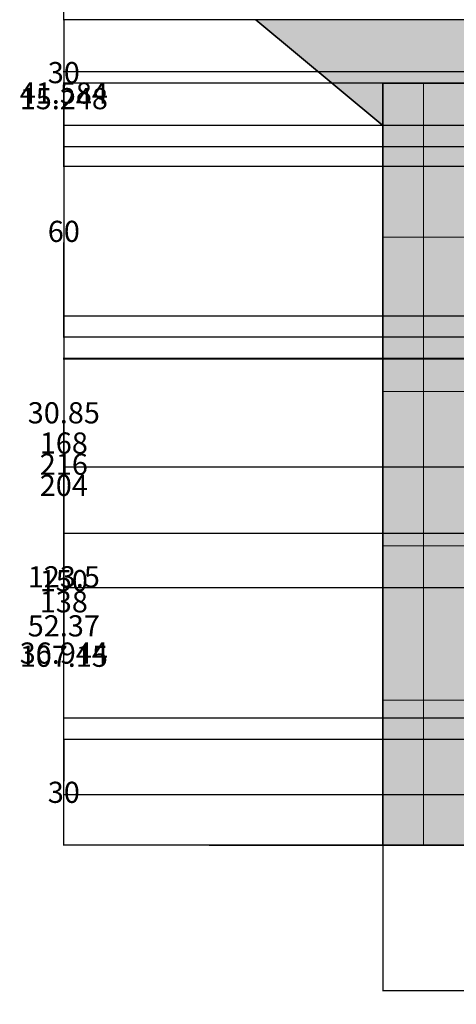
# Model space of a CAD drawing. Units: inches. Extents: x 148 to 1080, y 89 to 707.
# Tile 1 of 12: x 148 to 272, y 89 to 368. Entities that reach past the tile are written whole.
import ezdxf

# ---------------------------------------------------------------- set-up
doc = ezdxf.new("R2010")
doc.units = ezdxf.units.IN
doc.header["$MEASUREMENT"] = 0
for name, color, linetype, lineweight in [('A-ANNO-DIMS', 2, 'Continuous', 18), ('A-ELEV', 7, 'Continuous', 35), ('A-ELEV-PATT', 8, 'Continuous', 13)]:
    doc.layers.add(name, color=color, linetype=linetype, lineweight=lineweight)
doc.styles.get("Standard").update_dxf_attribs({"font": 'arial.ttf'})
doc.dimstyles.get("Standard").update_dxf_attribs({"dimtxt": 6, "dimasz": 0.18, "dimexe": 0.18, "dimexo": 0.0625, "dimgap": 0.09, "dimtad": 0, "dimtih": 1, "dimtoh": 1, "dimdec": 0, "dimzin": 0, "dimdsep": 46, "dimlunit": 3, "dimtxsty": 'Standard', "dimcen": 0.09, "dimadec": 0, "dimazin": 0, "dimtfac": 1, "dimtdec": 0, "dimtofl": 0, "dimtmove": 0, "dimatfit": 3, "dimfxl": 1, "dimtolj": 1, "dimtzin": 0, "dimarcsym": 0})

# ---------------------------------------------------------------- blocks, each defined once
blk = doc.blocks.new('*D1')
at = {"layer": 'A-ANNO-DIMS', "color": 0, "lineweight": -2, "transparency": 16777216}
for p, q in [((215.02, 662.01), (215.02, 703.28)), ((215.2, 703.1), (604.32, 703.1)), ((1006.77, 703.1), (617.65, 703.1)), ((1006.95, 338.01), (1006.95, 703.28))]:
    blk.add_line(p, q, dxfattribs=at)
at = {"layer": 'A-ANNO-DIMS', "color": 0, "transparency": 16777216}
for points in [[(215.2, 703.13), (215.2, 703.07), (215.02, 703.1)], [(1006.77, 703.13), (1006.77, 703.07), (1006.95, 703.1)]]:
    blk.add_solid(points, dxfattribs=at)
at = {"layer": 'Defpoints', "color": 0, "transparency": 16777216}
for p in [(1006.95, 703.1), (215.02, 661.95), (1006.95, 337.95)]:
    blk.add_point(p, dxfattribs=at)
at = {"layer": 'A-ANNO-DIMS', "color": 0, "transparency": 16777216, "insert": (610.98, 703.1), "char_height": 6, "attachment_point": 5}
blk.add_mtext('\\A1;792', dxfattribs=at)
blk = doc.blocks.new('*D2')
at = {"layer": 'A-ANNO-DIMS', "color": 0, "lineweight": -2, "transparency": 16777216}
for p, q in [((251.02, 133.88), (251.02, 92.62)), ((527.02, 133.88), (527.02, 92.62)), ((251.2, 92.8), (382.25, 92.8)), ((526.84, 92.8), (395.79, 92.8))]:
    blk.add_line(p, q, dxfattribs=at)
at = {"layer": 'A-ANNO-DIMS', "color": 0, "transparency": 16777216}
for points in [[(251.2, 92.83), (251.2, 92.77), (251.02, 92.8)], [(526.84, 92.83), (526.84, 92.77), (527.02, 92.8)]]:
    blk.add_solid(points, dxfattribs=at)
at = {"layer": 'Defpoints', "color": 0, "transparency": 16777216}
for p in [(251.02, 133.95), (527.02, 133.95), (527.02, 92.8)]:
    blk.add_point(p, dxfattribs=at)
at = {"layer": 'A-ANNO-DIMS', "color": 0, "transparency": 16777216, "insert": (389.02, 92.8), "char_height": 6, "attachment_point": 5}
blk.add_mtext('\\A1;276', dxfattribs=at)
blk = doc.blocks.new('*D22')
at = {"layer": 'A-ANNO-DIMS', "color": 0, "lineweight": -2, "transparency": 16777216}
for p, q in [((214.96, 400.95), (160.42, 400.95)), ((160.6, 400.77), (160.6, 387.6)), ((160.6, 368.13), (160.6, 381.29)), ((214.96, 367.95), (160.42, 367.95))]:
    blk.add_line(p, q, dxfattribs=at)
at = {"layer": 'A-ANNO-DIMS', "color": 0, "transparency": 16777216}
for points in [[(160.57, 400.77), (160.63, 400.77), (160.6, 400.95)], [(160.57, 368.13), (160.63, 368.13), (160.6, 367.95)]]:
    blk.add_solid(points, dxfattribs=at)
at = {"layer": 'Defpoints', "color": 0, "transparency": 16777216}
for p in [(215.02, 400.95), (160.6, 367.95), (215.02, 367.95)]:
    blk.add_point(p, dxfattribs=at)
at = {"layer": 'A-ANNO-DIMS', "color": 0, "transparency": 16777216, "insert": (160.6, 384.45), "char_height": 6, "attachment_point": 5}
blk.add_mtext('\\A1;33', dxfattribs=at)
blk = doc.blocks.new('*D23')
at = {"layer": 'A-ANNO-DIMS', "color": 0, "lineweight": -2, "transparency": 16777216}
for p, q in [((214.96, 367.95), (160.42, 367.95)), ((160.6, 367.77), (160.6, 356.1)), ((160.6, 338.13), (160.6, 349.79)), ((250.96, 337.95), (160.42, 337.95))]:
    blk.add_line(p, q, dxfattribs=at)
at = {"layer": 'A-ANNO-DIMS', "color": 0, "transparency": 16777216}
for points in [[(160.57, 367.77), (160.63, 367.77), (160.6, 367.95)], [(160.57, 338.13), (160.63, 338.13), (160.6, 337.95)]]:
    blk.add_solid(points, dxfattribs=at)
at = {"layer": 'Defpoints', "color": 0, "transparency": 16777216}
for p in [(215.02, 367.95), (160.6, 337.95), (251.02, 337.95)]:
    blk.add_point(p, dxfattribs=at)
at = {"layer": 'A-ANNO-DIMS', "color": 0, "transparency": 16777216, "insert": (160.6, 352.95), "char_height": 6, "attachment_point": 5}
blk.add_mtext('\\A1;30', dxfattribs=at)
blk = doc.blocks.new('*D24')
at = {"layer": 'A-ANNO-DIMS', "color": 0, "lineweight": -2, "transparency": 16777216}
for p, q in [((250.96, 337.95), (160.42, 337.95)), ((160.6, 337.77), (160.6, 239.1)), ((160.6, 134.13), (160.6, 232.79)), ((201.69, 133.95), (160.42, 133.95))]:
    blk.add_line(p, q, dxfattribs=at)
at = {"layer": 'A-ANNO-DIMS', "color": 0, "transparency": 16777216}
for points in [[(160.57, 337.77), (160.63, 337.77), (160.6, 337.95)], [(160.57, 134.13), (160.63, 134.13), (160.6, 133.95)]]:
    blk.add_solid(points, dxfattribs=at)
at = {"layer": 'Defpoints', "color": 0, "transparency": 16777216}
for p in [(251.02, 337.95), (160.6, 133.95), (201.75, 133.95)]:
    blk.add_point(p, dxfattribs=at)
at = {"layer": 'A-ANNO-DIMS', "color": 0, "transparency": 16777216, "insert": (160.6, 235.95), "char_height": 6, "attachment_point": 5}
blk.add_mtext('\\A1;204', dxfattribs=at)
blk = doc.blocks.new('*D28')
at = {"layer": 'A-ANNO-DIMS', "color": 0, "lineweight": -2, "transparency": 16777216}
for p, q in [((274.96, 331.95), (160.42, 331.95)), ((160.6, 331.77), (160.6, 251.1)), ((160.6, 164.13), (160.6, 244.79)), ((274.96, 163.95), (160.42, 163.95))]:
    blk.add_line(p, q, dxfattribs=at)
at = {"layer": 'A-ANNO-DIMS', "color": 0, "transparency": 16777216}
for points in [[(160.57, 331.77), (160.63, 331.77), (160.6, 331.95)], [(160.57, 164.13), (160.63, 164.13), (160.6, 163.95)]]:
    blk.add_solid(points, dxfattribs=at)
at = {"layer": 'Defpoints', "color": 0, "transparency": 16777216}
for p in [(160.6, 331.95), (275.02, 331.95), (275.02, 163.95)]:
    blk.add_point(p, dxfattribs=at)
at = {"layer": 'A-ANNO-DIMS', "color": 0, "transparency": 16777216, "insert": (160.6, 247.95), "char_height": 6, "attachment_point": 5}
blk.add_mtext('\\A1;168', dxfattribs=at)
blk = doc.blocks.new('*D29')
at = {"layer": 'A-ANNO-DIMS', "color": 0, "lineweight": -2, "transparency": 16777216}
for p, q in [((274.96, 163.95), (160.42, 163.95)), ((160.6, 163.77), (160.6, 152.1)), ((160.6, 134.13), (160.6, 145.79)), ((250.96, 133.95), (160.42, 133.95))]:
    blk.add_line(p, q, dxfattribs=at)
at = {"layer": 'A-ANNO-DIMS', "color": 0, "transparency": 16777216}
for points in [[(160.57, 163.77), (160.63, 163.77), (160.6, 163.95)], [(160.57, 134.13), (160.63, 134.13), (160.6, 133.95)]]:
    blk.add_solid(points, dxfattribs=at)
at = {"layer": 'Defpoints', "color": 0, "transparency": 16777216}
for p in [(275.02, 163.95), (160.6, 133.95), (251.02, 133.95)]:
    blk.add_point(p, dxfattribs=at)
at = {"layer": 'A-ANNO-DIMS', "color": 0, "transparency": 16777216, "insert": (160.6, 148.95), "char_height": 6, "attachment_point": 5}
blk.add_mtext('\\A1;30', dxfattribs=at)
blk = doc.blocks.new('*D30')
at = {"layer": 'A-ANNO-DIMS', "color": 0, "lineweight": -2, "transparency": 16777216}
for p, q in [((250.96, 349.95), (160.42, 349.95)), ((160.6, 349.77), (160.6, 245.1)), ((160.6, 134.13), (160.6, 238.79)), ((250.96, 133.95), (160.42, 133.95))]:
    blk.add_line(p, q, dxfattribs=at)
at = {"layer": 'A-ANNO-DIMS', "color": 0, "transparency": 16777216}
for points in [[(160.57, 349.77), (160.63, 349.77), (160.6, 349.95)], [(160.57, 134.13), (160.63, 134.13), (160.6, 133.95)]]:
    blk.add_solid(points, dxfattribs=at)
at = {"layer": 'Defpoints', "color": 0, "transparency": 16777216}
for p in [(251.02, 349.95), (160.6, 133.95), (251.02, 133.95)]:
    blk.add_point(p, dxfattribs=at)
at = {"layer": 'A-ANNO-DIMS', "color": 0, "transparency": 16777216, "insert": (160.6, 241.95), "char_height": 6, "attachment_point": 5}
blk.add_mtext('\\A1;216', dxfattribs=at)
blk = doc.blocks.new('*D32')
at = {"layer": 'A-ANNO-DIMS', "color": 0, "lineweight": -2, "transparency": 16777216}
for p, q in [((587, 271.77), (160.42, 271.77)), ((160.6, 271.59), (160.6, 213.18)), ((160.6, 148.46), (160.6, 206.87)), ((587, 148.28), (160.42, 148.28))]:
    blk.add_line(p, q, dxfattribs=at)
at = {"layer": 'A-ANNO-DIMS', "color": 0, "transparency": 16777216}
for points in [[(160.57, 271.59), (160.63, 271.59), (160.6, 271.77)], [(160.57, 148.46), (160.63, 148.46), (160.6, 148.28)]]:
    blk.add_solid(points, dxfattribs=at)
at = {"layer": 'Defpoints', "color": 0, "transparency": 16777216}
for p in [(160.6, 271.77), (587.06, 271.77), (587.06, 148.28)]:
    blk.add_point(p, dxfattribs=at)
at = {"layer": 'A-ANNO-DIMS', "color": 0, "transparency": 16777216, "insert": (160.6, 210.03), "char_height": 6, "attachment_point": 5}
blk.add_mtext('\\A1;123.5', dxfattribs=at)
blk = doc.blocks.new('*D34')
at = {"layer": 'A-ANNO-DIMS', "color": 0, "lineweight": -2, "transparency": 16777216}
for p, q in [((574.96, 283.95), (160.42, 283.95)), ((160.6, 283.77), (160.6, 212.1)), ((160.6, 134.13), (160.6, 205.79)), ((574.96, 133.95), (160.42, 133.95))]:
    blk.add_line(p, q, dxfattribs=at)
at = {"layer": 'A-ANNO-DIMS', "color": 0, "transparency": 16777216}
for points in [[(160.57, 283.77), (160.63, 283.77), (160.6, 283.95)], [(160.57, 134.13), (160.63, 134.13), (160.6, 133.95)]]:
    blk.add_solid(points, dxfattribs=at)
at = {"layer": 'Defpoints', "color": 0, "transparency": 16777216}
for p in [(575.02, 283.95), (160.6, 133.95), (575.02, 133.95)]:
    blk.add_point(p, dxfattribs=at)
at = {"layer": 'A-ANNO-DIMS', "color": 0, "transparency": 16777216, "insert": (160.6, 208.95), "char_height": 6, "attachment_point": 5}
blk.add_mtext('\\A1;150', dxfattribs=at)
blk = doc.blocks.new('*D38')
at = {"layer": 'A-ANNO-DIMS', "color": 0, "lineweight": -2, "transparency": 16777216}
for p, q in [((934.89, 271.95), (160.42, 271.95)), ((160.6, 271.77), (160.6, 206.1)), ((160.6, 134.13), (160.6, 199.79)), ((934.89, 133.95), (160.42, 133.95))]:
    blk.add_line(p, q, dxfattribs=at)
at = {"layer": 'A-ANNO-DIMS', "color": 0, "transparency": 16777216}
for points in [[(160.57, 271.77), (160.63, 271.77), (160.6, 271.95)], [(160.57, 134.13), (160.63, 134.13), (160.6, 133.95)]]:
    blk.add_solid(points, dxfattribs=at)
at = {"layer": 'Defpoints', "color": 0, "transparency": 16777216}
for p in [(934.95, 271.95), (160.6, 133.95), (934.95, 133.95)]:
    blk.add_point(p, dxfattribs=at)
at = {"layer": 'A-ANNO-DIMS', "color": 0, "transparency": 16777216, "insert": (160.6, 202.95), "char_height": 6, "attachment_point": 5}
blk.add_mtext('\\A1;138', dxfattribs=at)
blk = doc.blocks.new('*D39')
at = {"layer": 'A-ANNO-DIMS', "color": 0, "lineweight": -2, "transparency": 16777216}
for p, q in [((946.89, 337.95), (160.42, 337.95)), ((160.6, 337.77), (160.6, 311.1)), ((160.6, 278.13), (160.6, 304.79)), ((946.89, 277.95), (160.42, 277.95))]:
    blk.add_line(p, q, dxfattribs=at)
at = {"layer": 'A-ANNO-DIMS', "color": 0, "transparency": 16777216}
for points in [[(160.57, 337.77), (160.63, 337.77), (160.6, 337.95)], [(160.57, 278.13), (160.63, 278.13), (160.6, 277.95)]]:
    blk.add_solid(points, dxfattribs=at)
at = {"layer": 'Defpoints', "color": 0, "transparency": 16777216}
for p in [(160.6, 337.95), (946.95, 337.95), (946.95, 277.95)]:
    blk.add_point(p, dxfattribs=at)
at = {"layer": 'A-ANNO-DIMS', "color": 0, "transparency": 16777216, "insert": (160.6, 307.95), "char_height": 6, "attachment_point": 5}
blk.add_mtext('\\A1;60', dxfattribs=at)
blk = doc.blocks.new('*D42')
at = {"layer": 'A-ANNO-DIMS', "color": 0, "lineweight": -2, "transparency": 16777216}
for p, q in [((772.96, 367.95), (160.42, 367.95)), ((160.6, 367.77), (160.6, 350.31)), ((160.6, 326.54), (160.6, 344)), ((718.96, 326.36), (160.42, 326.36))]:
    blk.add_line(p, q, dxfattribs=at)
at = {"layer": 'A-ANNO-DIMS', "color": 0, "transparency": 16777216}
for points in [[(160.57, 367.77), (160.63, 367.77), (160.6, 367.95)], [(160.57, 326.54), (160.63, 326.54), (160.6, 326.36)]]:
    blk.add_solid(points, dxfattribs=at)
at = {"layer": 'Defpoints', "color": 0, "transparency": 16777216}
for p in [(773.02, 367.95), (160.6, 326.36), (719.02, 326.36)]:
    blk.add_point(p, dxfattribs=at)
at = {"layer": 'A-ANNO-DIMS', "color": 0, "transparency": 16777216, "insert": (160.6, 347.16), "char_height": 6, "attachment_point": 5}
blk.add_mtext('\\A1;41.584', dxfattribs=at)
blk = doc.blocks.new('*D43')
at = {"layer": 'A-ANNO-DIMS', "color": 0, "lineweight": -2, "transparency": 16777216}
for p, q in [((765.88, 241.1), (160.42, 241.1)), ((160.6, 240.92), (160.6, 190.68)), ((160.6, 134.13), (160.6, 184.37)), ((776.65, 133.95), (160.42, 133.95))]:
    blk.add_line(p, q, dxfattribs=at)
at = {"layer": 'A-ANNO-DIMS', "color": 0, "transparency": 16777216}
for points in [[(160.57, 240.92), (160.63, 240.92), (160.6, 241.1)], [(160.57, 134.13), (160.63, 134.13), (160.6, 133.95)]]:
    blk.add_solid(points, dxfattribs=at)
at = {"layer": 'Defpoints', "color": 0, "transparency": 16777216}
for p in [(765.95, 241.1), (160.6, 133.95), (776.71, 133.95)]:
    blk.add_point(p, dxfattribs=at)
at = {"layer": 'A-ANNO-DIMS', "color": 0, "transparency": 16777216, "insert": (160.6, 187.52), "char_height": 6, "attachment_point": 5}
blk.add_mtext('\\A1;107.15', dxfattribs=at)
blk = doc.blocks.new('*D49')
at = {"layer": 'A-ANNO-DIMS', "color": 0, "lineweight": -2, "transparency": 16777216}
for p, q in [((628.11, 353.2), (160.42, 353.2)), ((160.6, 353.02), (160.6, 348.73)), ((160.6, 338.13), (160.6, 342.42)), ((682.96, 337.95), (160.42, 337.95))]:
    blk.add_line(p, q, dxfattribs=at)
at = {"layer": 'A-ANNO-DIMS', "color": 0, "transparency": 16777216}
for points in [[(160.57, 353.02), (160.63, 353.02), (160.6, 353.2)], [(160.57, 338.13), (160.63, 338.13), (160.6, 337.95)]]:
    blk.add_solid(points, dxfattribs=at)
at = {"layer": 'Defpoints', "color": 0, "transparency": 16777216}
for p in [(628.17, 353.2), (160.6, 337.95), (683.02, 337.95)]:
    blk.add_point(p, dxfattribs=at)
at = {"layer": 'A-ANNO-DIMS', "color": 0, "transparency": 16777216, "insert": (160.6, 345.57), "char_height": 6, "attachment_point": 5}
blk.add_mtext('\\A1;15.248', dxfattribs=at)
blk = doc.blocks.new('*D80')
at = {"layer": 'A-ANNO-DIMS', "color": 0, "lineweight": -2, "transparency": 16777216}
for p, q in [((289.96, 222.32), (160.42, 222.32)), ((160.6, 222.14), (160.6, 199.29)), ((160.6, 170.13), (160.6, 192.98)), ((289.96, 169.95), (160.42, 169.95))]:
    blk.add_line(p, q, dxfattribs=at)
at = {"layer": 'A-ANNO-DIMS', "color": 0, "transparency": 16777216}
for points in [[(160.57, 222.14), (160.63, 222.14), (160.6, 222.32)], [(160.57, 170.13), (160.63, 170.13), (160.6, 169.95)]]:
    blk.add_solid(points, dxfattribs=at)
at = {"layer": 'Defpoints', "color": 0, "transparency": 16777216}
for p in [(160.6, 222.32), (290.02, 222.32), (290.02, 169.95)]:
    blk.add_point(p, dxfattribs=at)
at = {"layer": 'A-ANNO-DIMS', "color": 0, "transparency": 16777216, "insert": (160.6, 196.13), "char_height": 6, "attachment_point": 5}
blk.add_mtext('\\A1;52.37', dxfattribs=at)
blk = doc.blocks.new('*D81')
at = {"layer": 'A-ANNO-DIMS', "color": 0, "lineweight": -2, "transparency": 16777216}
for p, q in [((301.96, 206.89), (160.42, 206.89)), ((160.6, 206.71), (160.6, 191.57)), ((160.6, 170.13), (160.6, 185.26)), ((301.96, 169.95), (160.42, 169.95))]:
    blk.add_line(p, q, dxfattribs=at)
at = {"layer": 'A-ANNO-DIMS', "color": 0, "transparency": 16777216}
for points in [[(160.57, 206.71), (160.63, 206.71), (160.6, 206.89)], [(160.57, 170.13), (160.63, 170.13), (160.6, 169.95)]]:
    blk.add_solid(points, dxfattribs=at)
at = {"layer": 'Defpoints', "color": 0, "transparency": 16777216}
for p in [(160.6, 206.89), (302.02, 206.89), (302.02, 169.95)]:
    blk.add_point(p, dxfattribs=at)
at = {"layer": 'A-ANNO-DIMS', "color": 0, "transparency": 16777216, "insert": (160.6, 188.42), "char_height": 6, "attachment_point": 5}
blk.add_mtext('\\A1;36.944', dxfattribs=at)
blk = doc.blocks.new('*D102')
at = {"layer": 'A-ANNO-DIMS', "color": 0, "lineweight": -2, "transparency": 16777216}
for p, q in [((742.96, 271.95), (160.42, 271.95)), ((160.6, 271.77), (160.6, 259.68)), ((160.6, 241.28), (160.6, 253.37)), ((765.88, 241.1), (160.42, 241.1))]:
    blk.add_line(p, q, dxfattribs=at)
at = {"layer": 'A-ANNO-DIMS', "color": 0, "transparency": 16777216}
for points in [[(160.57, 271.77), (160.63, 271.77), (160.6, 271.95)], [(160.57, 241.28), (160.63, 241.28), (160.6, 241.1)]]:
    blk.add_solid(points, dxfattribs=at)
at = {"layer": 'Defpoints', "color": 0, "transparency": 16777216}
for p in [(160.6, 271.95), (743.02, 271.95), (765.95, 241.1)]:
    blk.add_point(p, dxfattribs=at)
at = {"layer": 'A-ANNO-DIMS', "color": 0, "transparency": 16777216, "insert": (160.6, 256.52), "char_height": 6, "attachment_point": 5}
blk.add_mtext('\\A1;30.85', dxfattribs=at)

msp = doc.modelspace()

# ---------------------------------------------------------------- hatches: boundary and pattern name
at = {"layer": 'A-ELEV-PATT'}
h = msp.add_hatch(color=256, dxfattribs=at)
h.dxf.hatch_style = 1
h.paths.add_polyline_path([(622.6005, 631.9474), (611.0199, 631.9474), (215.0199, 631.9474), (251.0199, 542.9352), (251.0199, 601.9474), (527.0199, 601.9474), (527.0199, 541.9474), (598.6005, 541.9474)])
h.paths.add_polyline_path([(558.5775, 608.9493, -1), (552.5775, 608.9493, -1)], flags=16)
h.paths.add_polyline_path([(586.7589, 556.0652, -1), (580.7589, 556.0652, -1)], flags=16)
h.paths.add_polyline_path([(635.0199, 631.9474), (622.6005, 631.9474), (598.6005, 541.9474), (611.0199, 541.9474)])
h.paths.add_polyline_path([(773.0199, 367.9474), (215.0199, 367.9474), (251.0199, 337.9474), (251.0199, 349.9474), (527.0199, 349.9474), (527.0199, 337.9474), (734.0628, 337.9474)])
h.paths.add_polyline_path([(631.1736, 353.1958, -1), (625.1736, 353.1958, -1)], flags=16)
h.paths.add_polyline_path([(729.9419, 354.8591, -1), (723.9419, 354.8591, -1)], flags=16)
h = msp.add_hatch(color=256, dxfattribs=at)
h.dxf.hatch_style = 1
h.paths.add_polyline_path([(527.0199, 349.9474), (395.0199, 349.9474), (395.0199, 271.2774), (527.0199, 272.3839)])
h.paths.add_polyline_path([(275.0199, 349.9474), (251.0199, 349.9474), (251.0199, 270.0704), (275.0199, 270.2716)])
h.paths.add_polyline_path([(743.0199, 337.9474), (734.0628, 337.9474), (719.0199, 326.3632), (719.0199, 277.9474), (743.0199, 277.9474)])
h.paths.add_polyline_path([(743.0199, 277.9474), (719.0199, 277.9474), (719.0199, 133.9474), (743.0199, 133.9474)])
h.paths.add_polyline_path([(734.0628, 337.9474), (719.0199, 337.9474), (719.0199, 326.3632)])
h = msp.add_hatch(dxfattribs=at)
h.set_pattern_fill('ANSI37', color=256, scale=350, angle=135)
h.paths.add_polyline_path([(527.0199, 349.9474), (395.0199, 349.9474), (395.0199, 163.9474), (275.0199, 163.9474), (275.0199, 349.9474), (251.0199, 349.9474), (251.0199, 133.9474), (527.0199, 133.9474)])
h = msp.add_hatch(color=256, dxfattribs=at)
h.dxf.hatch_style = 1
h.paths.add_polyline_path([(527.0199, 272.3839), (395.0199, 271.2774), (395.0199, 163.9474), (275.0199, 163.9474), (275.0199, 270.2716), (251.0199, 270.0704), (251.0199, 133.9474), (527.0199, 133.9474)])
h.paths.add_polyline_path([(1006.9492, 337.9474), (946.9492, 337.9474), (946.9492, 277.9474), (1006.9492, 277.9474)])
h.paths.add_polyline_path([(1006.9492, 277.9474), (946.9492, 277.9474), (946.9492, 133.9474), (1006.9492, 133.9474)])
h.paths.add_polyline_path([(946.9492, 337.9474), (743.0199, 337.9474), (743.0199, 277.9474), (946.9492, 277.9474)])

# ---------------------------------------------------------------- linework, layer by layer
at = {"layer": 'A-ELEV'}
for p, q in [((215.0199, 367.9474), (251.0199, 337.9474)), ((251.0199, 133.9474), (251.0199, 349.9474)), ((251.0199, 349.9474), (527.0199, 349.9474)), ((201.7492, 133.9474), (1023.175, 133.9474))]:
    msp.add_line(p, q, dxfattribs=at)

# ---------------------------------------------------------------- dimensions: what is measured, and where the dimension line sits
at = {"layer": 'A-ANNO-DIMS'}
for base, p1, p2, picture, middle in [((1006.9492, 703.0974), (215.0199, 661.9474), (1006.9492, 337.9474), '*D1', (610.9845, 703.0974)), ((527.0199, 92.7974), (251.0199, 133.9474), (527.0199, 133.9474), '*D2', (389.0199, 92.7974))]:
    dim = msp.add_linear_dim(base=base, p1=p1, p2=p2, dimstyle='Standard', override={"dimdec": 0, "dimlfac": 1, "dimrnd": 0, "dimzin": 0, "dimdsep": 46, "dimlunit": 2}, dxfattribs=at)
    dim.commit()
    dim.dimension.update_dxf_attribs({"geometry": picture, "text_midpoint": middle})
for base, p1, p2, override, picture, middle in [((160.5992, 367.9474), (215.0199, 400.9474), (215.0199, 367.9474), {"dimdec": 0, "dimlfac": 1, "dimrnd": 0, "dimzin": 0, "dimdsep": 46, "dimlunit": 2}, '*D22', (160.5992, 384.4474)), ((160.5992, 326.3632), (773.0199, 367.9474), (719.0199, 326.3632), {"dimdec": 3, "dimlfac": 1, "dimrnd": 0, "dimzin": 0, "dimdsep": 46, "dimlunit": 2}, '*D42', (160.5992, 347.1553)), ((160.5992, 337.9474), (215.0199, 367.9474), (251.0199, 337.9474), {"dimdec": 0, "dimlfac": 1, "dimrnd": 0, "dimzin": 0, "dimdsep": 46, "dimlunit": 2}, '*D23', (160.5992, 352.9474)), ((160.5992, 337.9474), (628.1736, 353.1958), (683.0199, 337.9474), {"dimdec": 3, "dimlfac": 1, "dimrnd": 0, "dimzin": 0, "dimdsep": 46, "dimlunit": 2}, '*D49', (160.5992, 345.5716)), ((160.5992, 133.9474), (251.0199, 349.9474), (251.0199, 133.9474), {"dimdec": 0, "dimlfac": 1, "dimrnd": 0, "dimzin": 0, "dimdsep": 46, "dimlunit": 2}, '*D30', (160.5992, 241.9474)), ((160.5992, 133.9474), (251.0199, 337.9474), (201.7492, 133.9474), {"dimdec": 0, "dimlfac": 1, "dimrnd": 0, "dimzin": 0, "dimdsep": 46, "dimlunit": 2}, '*D24', (160.5992, 235.9474)), ((160.5992, 337.9474), (946.9492, 277.9474), (946.9492, 337.9474), {"dimdec": 0, "dimlfac": 1, "dimrnd": 0, "dimzin": 0, "dimdsep": 46, "dimlunit": 2}, '*D39', (160.5992, 307.9474)), ((160.5992, 331.9474), (275.0199, 163.9474), (275.0199, 331.9474), {"dimdec": 0, "dimlfac": 1, "dimrnd": 0, "dimzin": 0, "dimdsep": 46, "dimlunit": 2}, '*D28', (160.5992, 247.9474)), ((160.5992, 133.9474), (575.0199, 283.9474), (575.0199, 133.9474), {"dimdec": 0, "dimlfac": 1, "dimrnd": 0, "dimzin": 0, "dimdsep": 46, "dimlunit": 2}, '*D34', (160.5992, 208.9474)), ((160.5992, 271.9474), (765.9474, 241.0996), (743.0199, 271.9474), {"dimdec": 2, "dimlfac": 1, "dimrnd": 0, "dimzin": 0, "dimdsep": 46, "dimlunit": 2}, '*D102', (160.5992, 256.5235)), ((160.5992, 271.7747), (587.0631, 148.2809), (587.0631, 271.7747), {"dimdec": 1, "dimlfac": 1, "dimrnd": 0, "dimzin": 0, "dimdsep": 46, "dimlunit": 2}, '*D32', (160.5992, 210.0278)), ((160.5992, 133.9474), (934.9492, 271.9474), (934.9492, 133.9474), {"dimdec": 0, "dimlfac": 1, "dimrnd": 0, "dimzin": 0, "dimdsep": 46, "dimlunit": 2}, '*D38', (160.5992, 202.9474)), ((160.5992, 133.9474), (765.9474, 241.0996), (776.713, 133.9474), {"dimdec": 2, "dimlfac": 1, "dimrnd": 0, "dimzin": 0, "dimdsep": 46, "dimlunit": 2}, '*D43', (160.5992, 187.5235)), ((160.5992, 222.3199), (290.0199, 169.9474), (290.0199, 222.3199), {"dimdec": 2, "dimlfac": 1, "dimrnd": 0, "dimzin": 0, "dimdsep": 46, "dimlunit": 2}, '*D80', (160.5992, 196.1336)), ((160.5992, 206.8913), (302.0199, 169.9474), (302.0199, 206.8913), {"dimdec": 3, "dimlfac": 1, "dimrnd": 0, "dimzin": 0, "dimdsep": 46, "dimlunit": 2}, '*D81', (160.5992, 188.4194)), ((160.5992, 133.9474), (275.0199, 163.9474), (251.0199, 133.9474), {"dimdec": 0, "dimlfac": 1, "dimrnd": 0, "dimzin": 0, "dimdsep": 46, "dimlunit": 2}, '*D29', (160.5992, 148.9474))]:
    dim = msp.add_linear_dim(base=base, p1=p1, p2=p2, angle=90, dimstyle='Standard', override=override, dxfattribs=at)
    dim.commit()
    dim.dimension.update_dxf_attribs({"geometry": picture, "text_midpoint": middle})

doc.saveas('drawing.dxf')
